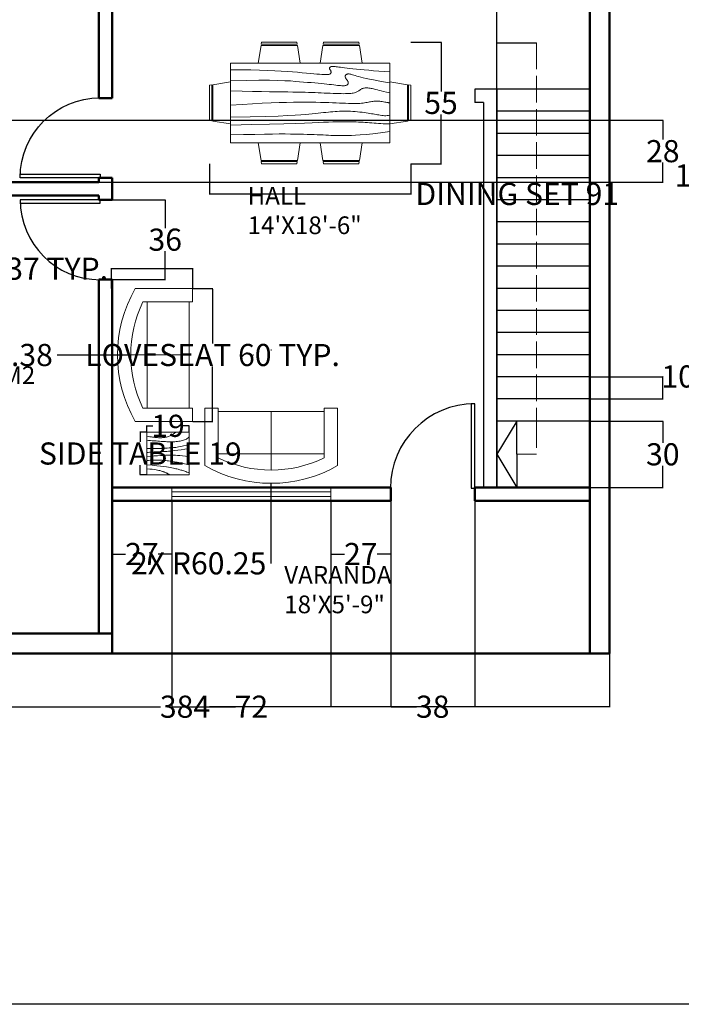
# Model space of a CAD drawing. Units: inches. Extents: x -16 to 1298, y 3 to 744.
# Tile 2 of 5: x 221 to 520, y 3 to 448. Entities that reach past the tile are written whole.
import ezdxf

# ---------------------------------------------------------------- set-up
doc = ezdxf.new("R2010")
doc.units = ezdxf.units.IN
doc.header["$MEASUREMENT"] = 0
doc.linetypes.add('ACAD_ISO02W100', pattern=[15, 12, -3])
for name, color, linetype, lineweight in [('A-ANNO-DIMS', 2, 'Continuous', 18), ('A-AREA-IDEN', 7, 'Continuous', 18), ('A-DOOR', 3, 'Continuous', 25), ('A-FLOR-STRS', 7, 'Continuous', 25), ('A-FLOR-STRS-PATH', 2, 'ACAD_ISO02W100', 13), ('A-FURN', 8, 'Continuous', 18), ('A-GLAZ', 4, 'Continuous', 18), ('A-WALL', 7, 'Continuous', 50)]:
    doc.layers.add(name, color=color, linetype=linetype, lineweight=lineweight)
doc.styles.get("Standard").update_dxf_attribs({"font": 'arial.ttf'})
doc.dimstyles.get("Standard").update_dxf_attribs({"dimtxt": 10, "dimasz": 0.18, "dimexe": 0.18, "dimexo": 0.0625, "dimgap": 0.09, "dimtad": 0, "dimtih": 1, "dimtoh": 1, "dimdec": 0, "dimzin": 0, "dimdsep": 46, "dimlunit": 3, "dimtxsty": 'Standard', "dimcen": 0.09, "dimadec": 0, "dimazin": 0, "dimtfac": 1, "dimtdec": 0, "dimtofl": 0, "dimtmove": 0, "dimatfit": 3, "dimfxl": 1, "dimtolj": 1, "dimtzin": 0, "dimarcsym": 0})

# ---------------------------------------------------------------- blocks, each defined once
blk = doc.blocks.new('Sofa - Roundback Loveseat 5 ft.')
for p, q in [((0, -32.44198), (0, -5.99998)), ((-24, -33.99998), (-24, -11.46958)), ((24.00004, -33.99998), (24.00004, -11.46958)), ((-23.9998, -13.38178), (23.99986, -13.38178)), ((-24, -32.44198), (24.00004, -32.44198))]:
    blk.add_line(p, q)
for points in [[(-24, -33.99998), (-30, -33.99998), (-30, -7.99998)], [(30.00004, -7.99998), (30.00004, -33.99998), (24.00004, -33.99998)]]:
    blk.add_lwpolyline(points)
for centre, radius, start, end in [((0, -60.24998), 60.24998, 60.13715, 119.8628), ((0, -61.38438), 55.38444, 64.32083, 115.6792)]:
    blk.add_arc(centre, radius, start, end)
blk = doc.blocks.new('Dining Set - 36 x 72 in.')
for p, q in [((-22, 27.5), (-22.1562, 26.50042)), ((-22, 27.5), (-6, 27.5)), ((-5.8437, 26.49966), (-6, 27.5)), ((6, 27.5), (5.8438, 26.50042)), ((6, 27.5), (22, 27.5)), ((22.1563, 26.49966), (22, 27.5)), ((-22.2343, 26.00059), (-23.4847, 17.99762)), ((-22.2304, 26), (-5.7608, 26)), ((-5.8416, 26.5), (-22.1534, 26.5)), ((-4.5152, 17.99762), (-5.7655, 25.99926)), ((5.7657, 26.00059), (4.5153, 17.99762)), ((5.7696, 26), (22.2392, 26)), ((22.1584, 26.5), (5.8466, 26.5)), ((23.4848, 17.99762), (22.2345, 25.99926)), ((36, 18), (-36, 18)), ((-36, 18), (-36, -18)), ((36, -18), (36, 18)), ((-44.0006, 8.23428), (-35.9976, 9.48474)), ((44.0006, 8.23428), (35.9976, 9.48474)), ((-45.5, 8), (-44.5004, 8.15617)), ((-45.5, 8), (-45.5, -8)), ((-44.5, -8.15843), (-44.5, 8.15338)), ((-44, 8.23041), (-44, -8.23915)), ((44, 8.23041), (44, -8.23915)), ((44.5, -8.15843), (44.5, 8.15338)), ((45.5, 8), (44.5005, 8.15617)), ((45.5, 8), (45.5, -8)), ((-44.4997, -8.15631), (-45.5, -8)), ((-35.9976, -9.48476), (-43.9993, -8.2345)), ((35.9976, -9.48476), (43.9993, -8.2345)), ((44.4997, -8.15631), (45.5, -8)), ((-36, -18), (36, -18)), ((-22.2343, -26.0006), (-23.4847, -17.99762)), ((-4.5152, -17.99762), (-5.7655, -25.99928)), ((5.7657, -26.0006), (4.5153, -17.99762)), ((23.4848, -17.99762), (22.2345, -25.99928)), ((-22.2304, -26), (-5.7608, -26)), ((-22, -27.5), (-22.1562, -26.50044)), ((-5.8416, -26.5), (-22.1534, -26.5)), ((-5.8437, -26.49967), (-6, -27.5)), ((5.7696, -26), (22.2392, -26)), ((6, -27.5), (5.8438, -26.50044)), ((22.1584, -26.5), (5.8466, -26.5)), ((22.1563, -26.49967), (22, -27.5)), ((-22, -27.5), (-6, -27.5)), ((6, -27.5), (22, -27.5))]:
    blk.add_line(p, q)
for points in [[(-36, 15), (-31.1772, 14.97754), (-26.8079, 14.91406), (-22.8538, 14.81543), (-19.276, 14.6875), (-16.0362, 14.53613), (-13.0957, 14.36718), (-10.4159, 14.18652), (-7.9583, 14), (-5.6904, 13.81315), (-3.6035, 13.63021), (-1.6954, 13.45508), (0.0365, 13.29166), (1.5945, 13.14388), (2.9811, 13.01562), (4.1988, 12.9108), (5.25, 12.83333), (6.1393, 12.78613), (6.8802, 12.76823), (7.4883, 12.77767), (7.9792, 12.8125), (8.3685, 12.87077), (8.6719, 12.95052), (8.9049, 13.0498), (9.0833, 13.16666), (9.2205, 13.29899), (9.3216, 13.44401), (9.3895, 13.59879), (9.4271, 13.76041), (9.4373, 13.92594), (9.4232, 14.09245), (9.3875, 14.257), (9.3333, 14.41666), (9.2638, 14.56917), (9.1836, 14.71484), (9.0975, 14.85465), (9.0104, 14.98958), (8.9272, 15.1206), (8.8529, 15.2487), (8.7922, 15.37483), (8.75, 15.5), (8.7305, 15.62467), (8.7344, 15.74739), (8.7617, 15.86621), (8.8125, 15.97916), (8.8867, 16.08431), (8.9844, 16.17968), (9.1055, 16.26334), (9.25, 16.33333), (9.4189, 16.38802), (9.6172, 16.42708), (9.8506, 16.45052), (10.125, 16.45833), (10.4463, 16.45052), (10.8203, 16.42708), (11.2529, 16.38802), (11.75, 16.33333), (12.3184, 16.26318), (12.9694, 16.17838), (13.7151, 16.07991), (14.5677, 15.96875), (15.5395, 15.84586), (16.6426, 15.71224), (17.8893, 15.56884), (19.2917, 15.41666), (20.859, 15.25667), (22.5879, 15.08984), (24.4721, 14.91715), (26.5052, 14.73958), (28.6809, 14.5581), (30.9929, 14.3737), (33.4347, 14.18733), (36, 14)], [(-36, 10), (-28.9766, 10.14274), (-23.1725, 10.20442), (-18.4241, 10.19775), (-14.5677, 10.13541), (-11.4399, 10.03011), (-8.877, 9.89453), (-6.7154, 9.74137), (-4.7917, 9.58333), (-2.9698, 9.43082), (-1.2246, 9.28515), (0.4415, 9.14534), (2.026, 9.01041), (3.5266, 8.87939), (4.9408, 8.7513), (6.266, 8.62516), (7.5, 8.5), (8.6411, 8.37549), (9.6914, 8.2539), (10.6538, 8.13818), (11.5312, 8.03125), (12.3267, 7.93603), (13.043, 7.85547), (13.6831, 7.79248), (14.25, 7.75), (14.7471, 7.7303), (15.1797, 7.73307), (15.5537, 7.75732), (15.875, 7.80208), (16.1494, 7.86637), (16.3828, 7.94922), (16.5811, 8.04964), (16.75, 8.16666), (16.8944, 8.29915), (17.0143, 8.44531), (17.1089, 8.60319), (17.1771, 8.77083), (17.218, 8.94629), (17.2305, 9.1276), (17.2137, 9.31282), (17.1667, 9.5), (17.0895, 9.6875), (16.987, 9.875), (16.8649, 10.0625), (16.7292, 10.25), (16.5856, 10.4375), (16.4401, 10.625), (16.2985, 10.8125), (16.1667, 11), (16.05, 11.18733), (15.9518, 11.3737), (15.8752, 11.5581), (15.8229, 11.73958), (15.798, 11.91715), (15.8034, 12.08984), (15.842, 12.25667), (15.9167, 12.41666), (16.0295, 12.56836), (16.1784, 12.70833), (16.3605, 12.83268), (16.5729, 12.9375), (16.8127, 13.01888), (17.0768, 13.07291), (17.3625, 13.0957), (17.6667, 13.08333), (17.9894, 13.03312), (18.3418, 12.94726), (18.7382, 12.82918), (19.1927, 12.68229), (19.7195, 12.51001), (20.3327, 12.31575), (21.0465, 12.10294), (21.875, 11.875), (22.8357, 11.63354), (23.959, 11.37304), (25.2786, 11.08618), (26.8282, 10.76562), (28.6414, 10.40405), (30.752, 9.99414), (33.1936, 9.52856), (36, 9)], [(-36, 5.5), (-30.7157, 5.3348), (-26.069, 5.20963), (-21.9946, 5.11767), (-18.4271, 5.05208), (-15.3009, 5.00602), (-12.5508, 4.97265), (-10.1112, 4.94515), (-7.9167, 4.91666), (-5.909, 4.88167), (-4.0586, 4.83984), (-2.3429, 4.79215), (-0.7396, 4.73958), (0.7739, 4.6831), (2.22, 4.6237), (3.6213, 4.56233), (5, 4.5), (6.373, 4.43782), (7.7344, 4.3776), (9.0723, 4.32129), (10.375, 4.27083), (11.6309, 4.22819), (12.8281, 4.19531), (13.9551, 4.17415), (15, 4.16666), (15.954, 4.17448), (16.819, 4.19791), (17.6001, 4.23698), (18.3021, 4.29166), (18.9299, 4.36198), (19.4883, 4.44791), (19.9823, 4.54948), (20.4167, 4.66666), (20.7969, 4.79899), (21.1302, 4.94401), (21.4245, 5.09879), (21.6875, 5.26041), (21.9271, 5.42594), (22.1511, 5.59245), (22.3672, 5.757), (22.5834, 5.91666), (22.8065, 6.06868), (23.0404, 6.21093), (23.2879, 6.34147), (23.5521, 6.45833), (23.8358, 6.55957), (24.142, 6.64323), (24.4735, 6.70735), (24.8334, 6.75), (25.2235, 6.76969), (25.642, 6.76692), (26.0858, 6.74267), (26.5521, 6.69791), (27.0379, 6.63362), (27.5404, 6.55078), (28.0565, 6.45036), (28.5834, 6.33333), (29.1242, 6.19987), (29.7071, 6.04687), (30.3661, 5.87044), (31.1354, 5.66666), (32.0493, 5.43164), (33.142, 5.16146), (34.4475, 4.85221), (36, 4.5)], [(-36, -1), (-30.7915, -0.6591), (-26.0195, -0.38216), (-21.6519, -0.16284), (-17.6563, 0.00521), (-14.0005, 0.12833), (-10.6523, 0.21289), (-7.5796, 0.26522), (-4.75, 0.29166), (-2.134, 0.29793), (0.2878, 0.28711), (2.5317, 0.26163), (4.6146, 0.22396), (6.5529, 0.17651), (8.3633, 0.12174), (10.0623, 0.06209), (11.6667, 0), (13.1899, -0.06201), (14.6341, -0.1211), (15.9982, -0.17432), (17.2813, -0.21875), (18.4823, -0.25147), (19.6003, -0.26953), (20.6343, -0.27002), (21.5834, -0.25), (22.4481, -0.20768), (23.2357, -0.14584), (23.9549, -0.06836), (24.6146, 0.02083), (25.2235, 0.11784), (25.7904, 0.21875), (26.3241, 0.31966), (26.8334, 0.41666), (27.3265, 0.50618), (27.8099, 0.58593), (28.2894, 0.65397), (28.7709, 0.70833), (29.2601, 0.74707), (29.763, 0.76823), (30.2855, 0.76985), (30.8334, 0.75), (31.4088, 0.70784), (31.9994, 0.64713), (32.589, 0.57275), (33.1615, 0.48958), (33.7008, 0.4025), (34.1908, 0.3164), (34.6153, 0.23616), (34.9584, 0.16666), (35.2099, 0.11165), (35.3848, 0.07031), (35.504, 0.04069), (35.5886, 0.02083), (35.6594, 0.00879), (35.7377, 0.0026), (35.8442, 0.00032), (36, 0)], [(-36, -6.5), (-27.1843, -6.31267), (-20.084, -6.1263), (-14.469, -5.9419), (-10.1094, -5.76042), (-6.7752, -5.58285), (-4.2363, -5.41016), (-2.2629, -5.24333), (-0.625, -5.08334), (0.8708, -4.93099), (2.2715, -4.78646), (3.5872, -4.64974), (4.8281, -4.52084), (6.0046, -4.39974), (7.127, -4.28646), (8.2053, -4.18099), (9.25, -4.08334), (10.2705, -3.99382), (11.2734, -3.91407), (12.2647, -3.84603), (13.25, -3.79167), (14.2354, -3.75293), (15.2266, -3.73177), (16.2295, -3.73015), (17.25, -3.75), (18.2912, -3.79248), (19.3451, -3.85547), (20.4009, -3.93604), (21.4479, -4.03125), (22.4754, -4.13819), (23.4727, -4.25391), (24.4289, -4.37549), (25.3334, -4.5), (26.1785, -4.62492), (26.9694, -4.74935), (27.7145, -4.87281), (28.4219, -4.99479), (29.1, -5.11483), (29.7572, -5.23242), (30.4016, -5.34709), (31.0417, -5.45834), (31.6837, -5.56437), (32.3262, -5.65821), (32.9658, -5.73153), (33.599, -5.77604), (34.2224, -5.78345), (34.8327, -5.74545), (35.4264, -5.65373), (36, -5.5)], [(-36, -10), (-26.4022, -9.81299), (-18.4675, -9.62891), (-11.9839, -9.45069), (-6.7396, -9.28125), (-2.5226, -9.12354), (0.8789, -8.98047), (3.6769, -8.85498), (6.0833, -8.75), (8.2767, -8.66765), (10.3021, -8.60677), (12.1712, -8.56543), (13.8958, -8.54167), (15.4876, -8.53353), (16.9583, -8.53907), (18.3197, -8.55632), (19.5834, -8.58334), (20.7616, -8.61841), (21.8685, -8.66081), (22.9188, -8.71004), (23.9271, -8.76563), (24.9081, -8.82707), (25.8763, -8.89388), (26.8465, -8.96558), (27.8334, -9.04167), (28.8474, -9.12118), (29.8828, -9.20117), (30.93, -9.27824), (31.9792, -9.34896), (33.0205, -9.40991), (34.0443, -9.45768), (35.0407, -9.48885), (36, -9.5)], [(-36, -14.5), (-30.0881, -14.33513), (-25.0332, -14.21224), (-20.7312, -14.12647), (-17.0781, -14.07292), (-13.97, -14.04671), (-11.3027, -14.04297), (-8.9724, -14.05681), (-6.875, -14.08334), (-4.9224, -14.11833), (-3.0905, -14.16016), (-1.3709, -14.20785), (0.2448, -14.26042), (1.7647, -14.3169), (3.1973, -14.3763), (4.5507, -14.43767), (5.8333, -14.5), (7.0554, -14.5621), (8.235, -14.62175), (9.3922, -14.67652), (10.5469, -14.72396), (11.7192, -14.76164), (12.929, -14.78711), (14.1965, -14.79794), (15.5417, -14.79167), (16.9933, -14.76424), (18.6152, -14.70508), (20.4804, -14.60197), (22.6615, -14.44271), (25.2312, -14.21509), (28.2624, -13.9069), (31.8277, -13.50594), (36, -13)]]:
    blk.add_lwpolyline(points)
blk = doc.blocks.new('*U8')
for p, q in [((0, 0), (0, -6)), ((-40, 0), (-40, -6))]:
    blk.add_line(p, q)
blk.add_lwpolyline([(0, 0), (0, 40), (-1.75, 40), (-1.75, 0)], close=True)
blk.add_arc((0, 0), 40, 90, 180)
blk = doc.blocks.new('Table - Square Woodgrain 42 x 42 in.')
blk.add_line((0, -42), (42, -42))
for points in [[(0, -4), (1.704, -4.2172), (3.2358, -4.4188), (4.615, -4.604), (5.8615, -4.7721), (6.9951, -4.9224), (8.0357, -5.0541), (9.0031, -5.1667), (9.9171, -5.2594), (10.7951, -5.3316), (11.6445, -5.3836), (12.4702, -5.4157), (13.277, -5.4283), (14.0698, -5.4217), (14.8535, -5.3964), (15.6331, -5.3526), (16.4133, -5.2908), (17.1986, -5.2103), (17.9913, -5.1062), (18.793, -4.9727), (19.6056, -4.8038), (20.4307, -4.5937), (21.2701, -4.3365), (22.1256, -4.0262), (22.9989, -3.6571), (23.888, -3.2272), (24.7756, -2.7516), (25.6408, -2.2491), (26.4624, -1.7387), (27.2195, -1.2395), (27.891, -0.7703), (28.456, -0.3501), (28.8934, 0.002)], [(0, -42), (0, 0), (42, 0), (42, -42)], [(0, -8), (1.8203, -8.1001), (3.6741, -8.2149), (5.5411, -8.3408), (7.4011, -8.4741), (9.2339, -8.6112), (11.0193, -8.7484), (12.7371, -8.8821), (14.3671, -9.0086), (15.8954, -9.1246), (17.3337, -9.2278), (18.6997, -9.3159), (20.0116, -9.387), (21.2871, -9.4389), (22.5442, -9.4696), (23.8008, -9.477), (25.0749, -9.459), (26.3791, -9.4137), (27.7049, -9.3403), (29.0383, -9.2382), (30.3655, -9.1068), (31.6728, -8.9455), (32.9461, -8.7535), (34.1717, -8.5304), (35.3358, -8.2756), (36.4268, -7.9863), (37.443, -7.6521), (38.3849, -7.2603), (39.253, -6.7986), (40.048, -6.2542), (40.7705, -5.6147), (41.421, -4.8674), (42, -4)], [(42, -12), (39.1784, -12.8621), (36.4519, -13.5654), (33.8246, -14.1294), (31.3004, -14.5731), (28.8832, -14.9161), (26.577, -15.1775), (24.3858, -15.3768), (22.3136, -15.5332), (20.3622, -15.6632), (18.5254, -15.7718), (16.7947, -15.8612), (15.1618, -15.9338), (13.6183, -15.9916), (12.1558, -16.0369), (10.7659, -16.0718), (9.4403, -16.0987), (8.1703, -16.1191), (6.9461, -16.1325), (5.7577, -16.1377), (4.595, -16.1335), (3.4479, -16.1188), (2.3064, -16.0924), (1.1604, -16.0532), (0, -16)], [(42, -16), (37.6529, -16.7365), (33.8802, -17.329), (30.6179, -17.7961), (27.8015, -18.1561), (25.3668, -18.4275), (23.2497, -18.6288), (21.3859, -18.7785), (19.7111, -18.8949), (18.1693, -18.9939), (16.7375, -19.0795), (15.401, -19.1534), (14.1449, -19.217), (12.9544, -19.2717), (11.8148, -19.3191), (10.7113, -19.3606), (9.6291, -19.3976), (8.5534, -19.4323), (7.47, -19.4689), (6.3643, -19.5122), (5.222, -19.5672), (4.0288, -19.6386), (2.7703, -19.7313), (1.4321, -19.8501), (0, -20)], [(0, -24), (3.9243, -23.6805), (7.4766, -23.4138), (10.6891, -23.1954), (13.5943, -23.0205), (16.2247, -22.8847), (18.6125, -22.7832), (20.7903, -22.7116), (22.7903, -22.6651), (24.6563, -22.642), (26.4764, -22.6507), (28.35, -22.7024), (30.3766, -22.8084), (32.6555, -22.98), (35.2861, -23.2283), (38.3678, -23.5645), (42, -24)], [(42, -32), (37.392, -31.017), (33.4585, -30.2231), (30.1291, -29.5949), (27.3334, -29.109), (25.0009, -28.742), (23.0612, -28.4707), (21.4439, -28.2716), (20.0786, -28.1215), (18.8998, -28.0002), (17.8609, -27.9014), (16.9206, -27.8219), (16.0371, -27.7588), (15.1691, -27.709), (14.2748, -27.6693), (13.3128, -27.6368), (12.2415, -27.6083), (11.0295, -27.5824), (9.6867, -27.5643), (8.233, -27.5608), (6.6884, -27.5787), (5.0728, -27.6248), (3.4062, -27.7058), (1.7086, -27.8286), (0, -28)], [(0, -32), (5.4026, -32.5358), (9.9494, -33.019), (13.7424, -33.4553), (16.8834, -33.8505), (19.4743, -34.2106), (21.6171, -34.5413), (23.4136, -34.8486), (24.9657, -35.1382), (26.3614, -35.4156), (27.6332, -35.6841), (28.7995, -35.9467), (29.8788, -36.2064), (30.8897, -36.4661), (31.8507, -36.7288), (32.7802, -36.9973), (33.6968, -37.2747), (34.6175, -37.5635), (35.5531, -37.8651), (36.5128, -38.1805), (37.506, -38.5108), (38.5421, -38.8568), (39.6302, -39.2197), (40.7797, -39.6004), (42, -40)], [(0, -36), (3.0098, -36.2857), (5.5354, -36.5643), (7.6368, -36.8359), (9.374, -37.1009), (10.807, -37.3597), (11.9957, -37.6126), (13.0002, -37.8599), (13.8804, -38.102), (14.6874, -38.3393), (15.4365, -38.5729), (16.1338, -38.8041), (16.7858, -39.0341), (17.3987, -39.264), (17.9787, -39.4952), (18.5322, -39.7288), (19.0655, -39.9662), (19.5832, -40.2081), (20.0842, -40.4544), (20.5657, -40.7046), (21.0249, -40.9581), (21.459, -41.2144), (21.8653, -41.4731), (22.2409, -41.7335), (22.5831, -41.9951)]]:
    blk.add_lwpolyline(points)
blk = doc.blocks.new('*D32')
at = {"layer": 'A-ANNO-DIMS', "color": 0, "lineweight": -2, "transparency": 16777216}
for p, q in [((299.2, 326.87), (308.32, 326.87)), ((308.14, 326.69), (308.14, 302.13)), ((308.14, 267.05), (308.14, 291.61)), ((299.2, 266.87), (308.32, 266.87))]:
    blk.add_line(p, q, dxfattribs=at)
at = {"layer": 'A-ANNO-DIMS', "color": 0, "transparency": 16777216}
for points in [[(308.11, 326.69), (308.17, 326.69), (308.14, 326.87)], [(308.11, 267.05), (308.17, 267.05), (308.14, 266.87)]]:
    blk.add_solid(points, dxfattribs=at)
at = {"layer": 'Defpoints', "color": 0, "transparency": 16777216}
for p in [(299.14, 326.87), (308.14, 326.87), (299.14, 266.87)]:
    blk.add_point(p, dxfattribs=at)
at = {"layer": 'A-ANNO-DIMS', "color": 0, "transparency": 16777216, "insert": (308.14, 296.87), "char_height": 10, "attachment_point": 5}
blk.add_mtext('\\A1;LOVESEAT 60 TYP.', dxfattribs=at)
blk = doc.blocks.new('*D33')
at = {"layer": 'A-ANNO-DIMS', "color": 0, "lineweight": -2, "transparency": 16777216}
for p, q in [((262.47, 335.87), (262.29, 335.87)), ((262.47, 326.93), (262.47, 336.05)), ((298.96, 335.87), (262.65, 335.87)), ((299.14, 326.93), (299.14, 336.05))]:
    blk.add_line(p, q, dxfattribs=at)
at = {"layer": 'A-ANNO-DIMS', "color": 0, "transparency": 16777216}
for points in [[(262.65, 335.9), (262.65, 335.84), (262.47, 335.87)], [(298.96, 335.9), (298.96, 335.84), (299.14, 335.87)]]:
    blk.add_solid(points, dxfattribs=at)
at = {"layer": 'Defpoints', "color": 0, "transparency": 16777216}
for p in [(262.47, 335.87), (262.47, 326.87), (299.14, 326.87)]:
    blk.add_point(p, dxfattribs=at)
at = {"layer": 'A-ANNO-DIMS', "color": 0, "transparency": 16777216, "insert": (237.87, 335.87), "char_height": 10, "attachment_point": 5}
blk.add_mtext('\\A1;37 TYP.', dxfattribs=at)
blk = doc.blocks.new('*D34')
at = {"layer": 'A-ANNO-DIMS', "color": 0, "lineweight": -2, "transparency": 16777216}
for p, q in [((278.28, 261.98), (275.28, 261.98)), ((275.46, 261.8), (275.46, 257.61)), ((275.46, 242.9), (275.46, 247.09)), ((278.28, 242.72), (275.28, 242.72))]:
    blk.add_line(p, q, dxfattribs=at)
at = {"layer": 'A-ANNO-DIMS', "color": 0, "transparency": 16777216}
for points in [[(275.43, 261.8), (275.49, 261.8), (275.46, 261.98)], [(275.43, 242.9), (275.49, 242.9), (275.46, 242.72)]]:
    blk.add_solid(points, dxfattribs=at)
at = {"layer": 'Defpoints', "color": 0, "transparency": 16777216}
for p in [(275.46, 261.98), (278.35, 261.98), (278.35, 242.72)]:
    blk.add_point(p, dxfattribs=at)
at = {"layer": 'A-ANNO-DIMS', "color": 0, "transparency": 16777216, "insert": (275.46, 252.35), "char_height": 10, "attachment_point": 5}
blk.add_mtext('\\A1;SIDE TABLE 19', dxfattribs=at)
blk = doc.blocks.new('*D35')
at = {"layer": 'A-ANNO-DIMS', "color": 0, "lineweight": -2, "transparency": 16777216}
for p, q in [((278.35, 262.04), (278.35, 265.05)), ((278.53, 264.87), (281.18, 264.87)), ((297.42, 264.87), (294.77, 264.87)), ((297.6, 262.04), (297.6, 265.05))]:
    blk.add_line(p, q, dxfattribs=at)
at = {"layer": 'A-ANNO-DIMS', "color": 0, "transparency": 16777216}
for points in [[(278.53, 264.9), (278.53, 264.84), (278.35, 264.87)], [(297.42, 264.9), (297.42, 264.84), (297.6, 264.87)]]:
    blk.add_solid(points, dxfattribs=at)
at = {"layer": 'Defpoints', "color": 0, "transparency": 16777216}
for p in [(297.6, 264.87), (278.35, 261.98), (297.6, 261.98)]:
    blk.add_point(p, dxfattribs=at)
at = {"layer": 'A-ANNO-DIMS', "color": 0, "transparency": 16777216, "insert": (287.97, 264.87), "char_height": 10, "attachment_point": 5}
blk.add_mtext('\\A1;19', dxfattribs=at)
blk = doc.blocks.new('*D36')
at = {"layer": 'A-ANNO-DIMS', "color": 0, "lineweight": -2, "transparency": 16777216}
for p, q in [((306.79, 383.23), (306.79, 369.47)), ((397.79, 383.23), (397.79, 369.47)), ((306.97, 369.65), (397.61, 369.65)), ((397.79, 369.65), (397.97, 369.65))]:
    blk.add_line(p, q, dxfattribs=at)
at = {"layer": 'A-ANNO-DIMS', "color": 0, "transparency": 16777216}
for points in [[(306.97, 369.68), (306.97, 369.62), (306.79, 369.65)], [(397.61, 369.68), (397.61, 369.62), (397.79, 369.65)]]:
    blk.add_solid(points, dxfattribs=at)
at = {"layer": 'Defpoints', "color": 0, "transparency": 16777216}
for p in [(306.79, 383.3), (397.79, 383.3), (397.79, 369.65)]:
    blk.add_point(p, dxfattribs=at)
at = {"layer": 'A-ANNO-DIMS', "color": 0, "transparency": 16777216, "insert": (445.92, 369.65), "char_height": 10, "attachment_point": 5}
blk.add_mtext('\\A1;DINING SET 91', dxfattribs=at)
blk = doc.blocks.new('*D37')
at = {"layer": 'A-ANNO-DIMS', "color": 0, "lineweight": -2, "transparency": 16777216}
for p, q in [((397.85, 438.3), (411.62, 438.3)), ((411.44, 438.12), (411.44, 415.97)), ((411.44, 383.48), (411.44, 405.62)), ((397.85, 383.3), (411.62, 383.3))]:
    blk.add_line(p, q, dxfattribs=at)
at = {"layer": 'A-ANNO-DIMS', "color": 0, "transparency": 16777216}
for points in [[(411.41, 438.12), (411.47, 438.12), (411.44, 438.3)], [(411.41, 383.48), (411.47, 383.48), (411.44, 383.3)]]:
    blk.add_solid(points, dxfattribs=at)
at = {"layer": 'Defpoints', "color": 0, "transparency": 16777216}
for p in [(397.79, 438.3), (411.44, 438.3), (397.79, 383.3)]:
    blk.add_point(p, dxfattribs=at)
at = {"layer": 'A-ANNO-DIMS', "color": 0, "transparency": 16777216, "insert": (411.44, 410.8), "char_height": 10, "attachment_point": 5}
blk.add_mtext('\\A1;55', dxfattribs=at)
blk = doc.blocks.new('*D40')
at = {"layer": 'A-ANNO-DIMS', "color": 0, "lineweight": -2, "transparency": 16777216}
for p, q in [((103.68, 161.93), (103.68, 137.76)), ((487.68, 161.93), (487.68, 137.76)), ((103.86, 137.94), (284.56, 137.94)), ((487.5, 137.94), (306.79, 137.94))]:
    blk.add_line(p, q, dxfattribs=at)
at = {"layer": 'A-ANNO-DIMS', "color": 0, "transparency": 16777216}
for points in [[(103.86, 137.97), (103.86, 137.91), (103.68, 137.94)], [(487.5, 137.97), (487.5, 137.91), (487.68, 137.94)]]:
    blk.add_solid(points, dxfattribs=at)
at = {"layer": 'Defpoints', "color": 0, "transparency": 16777216}
for p in [(103.68, 161.99), (487.68, 161.99), (487.68, 137.94)]:
    blk.add_point(p, dxfattribs=at)
at = {"layer": 'A-ANNO-DIMS', "color": 0, "transparency": 16777216, "insert": (295.68, 137.94), "char_height": 10, "attachment_point": 5}
blk.add_mtext('\\A1;384', dxfattribs=at)
blk = doc.blocks.new('*D42')
at = {"layer": 'A-ANNO-DIMS', "color": 0, "lineweight": -2, "transparency": 16777216}
for p, q in [((436.68, 237.05), (436.68, 618.22)), ((436.86, 618.04), (450.27, 618.04)), ((478.5, 618.04), (465.08, 618.04)), ((478.68, 237.05), (478.68, 618.22))]:
    blk.add_line(p, q, dxfattribs=at)
at = {"layer": 'A-ANNO-DIMS', "color": 0, "transparency": 16777216}
for points in [[(436.86, 618.07), (436.86, 618.01), (436.68, 618.04)], [(478.5, 618.07), (478.5, 618.01), (478.68, 618.04)]]:
    blk.add_solid(points, dxfattribs=at)
at = {"layer": 'Defpoints', "color": 0, "transparency": 16777216}
for p in [(478.68, 618.04), (436.68, 236.99), (478.68, 236.99)]:
    blk.add_point(p, dxfattribs=at)
at = {"layer": 'A-ANNO-DIMS', "color": 0, "transparency": 16777216, "insert": (457.68, 618.04), "char_height": 10, "attachment_point": 5}
blk.add_mtext('\\A1;42', dxfattribs=at)
blk = doc.blocks.new('*D43')
at = {"layer": 'A-ANNO-DIMS', "color": 0, "lineweight": -2, "transparency": 16777216}
for p, q in [((478.74, 266.99), (511.91, 266.99)), ((511.73, 266.81), (511.73, 257.19)), ((511.73, 237.17), (511.73, 246.79)), ((478.74, 236.99), (511.91, 236.99))]:
    blk.add_line(p, q, dxfattribs=at)
at = {"layer": 'A-ANNO-DIMS', "color": 0, "transparency": 16777216}
for points in [[(511.7, 266.81), (511.76, 266.81), (511.73, 266.99)], [(511.7, 237.17), (511.76, 237.17), (511.73, 236.99)]]:
    blk.add_solid(points, dxfattribs=at)
at = {"layer": 'Defpoints', "color": 0, "transparency": 16777216}
for p in [(478.68, 266.99), (511.73, 266.99), (478.68, 236.99)]:
    blk.add_point(p, dxfattribs=at)
at = {"layer": 'A-ANNO-DIMS', "color": 0, "transparency": 16777216, "insert": (511.73, 251.99), "char_height": 10, "attachment_point": 5}
blk.add_mtext('\\A1;30', dxfattribs=at)
blk = doc.blocks.new('*D44')
at = {"layer": 'A-ANNO-DIMS', "color": 0, "lineweight": -2, "transparency": 16777216}
for p, q in [((478.74, 286.99), (511.91, 286.99)), ((511.73, 286.99), (511.73, 287.17)), ((511.73, 287.17), (511.91, 287.17)), ((511.73, 277.17), (511.73, 286.81)), ((478.74, 276.99), (511.91, 276.99))]:
    blk.add_line(p, q, dxfattribs=at)
at = {"layer": 'A-ANNO-DIMS', "color": 0, "transparency": 16777216}
for points in [[(511.7, 286.81), (511.76, 286.81), (511.73, 286.99)], [(511.7, 277.17), (511.76, 277.17), (511.73, 276.99)]]:
    blk.add_solid(points, dxfattribs=at)
at = {"layer": 'Defpoints', "color": 0, "transparency": 16777216}
for p in [(478.68, 286.99), (511.73, 286.99), (478.68, 276.99)]:
    blk.add_point(p, dxfattribs=at)
at = {"layer": 'A-ANNO-DIMS', "color": 0, "transparency": 16777216, "insert": (518.67, 287.17), "char_height": 10, "attachment_point": 5}
blk.add_mtext('\\A1;10', dxfattribs=at)
blk = doc.blocks.new('*D49')
at = {"layer": 'A-ANNO-DIMS', "color": 0, "lineweight": -2, "transparency": 16777216}
for p, q in [((262.68, 230.93), (262.68, 206.76)), ((289.68, 230.93), (289.68, 206.76)), ((262.86, 206.94), (268.84, 206.94)), ((289.5, 206.94), (283.51, 206.94))]:
    blk.add_line(p, q, dxfattribs=at)
at = {"layer": 'A-ANNO-DIMS', "color": 0, "transparency": 16777216}
for points in [[(262.86, 206.97), (262.86, 206.91), (262.68, 206.94)], [(289.5, 206.97), (289.5, 206.91), (289.68, 206.94)]]:
    blk.add_solid(points, dxfattribs=at)
at = {"layer": 'Defpoints', "color": 0, "transparency": 16777216}
for p in [(262.68, 230.99), (289.68, 230.99), (262.68, 206.94)]:
    blk.add_point(p, dxfattribs=at)
at = {"layer": 'A-ANNO-DIMS', "color": 0, "transparency": 16777216, "insert": (276.18, 206.94), "char_height": 10, "attachment_point": 5}
blk.add_mtext('\\A1;27', dxfattribs=at)
blk = doc.blocks.new('*D50')
at = {"layer": 'A-ANNO-DIMS', "color": 0, "lineweight": -2, "transparency": 16777216}
for p, q in [((289.68, 230.93), (289.68, 137.76)), ((361.68, 230.93), (361.68, 137.76)), ((289.86, 137.94), (318.52, 137.94)), ((361.5, 137.94), (332.84, 137.94))]:
    blk.add_line(p, q, dxfattribs=at)
at = {"layer": 'A-ANNO-DIMS', "color": 0, "transparency": 16777216}
for points in [[(289.86, 137.97), (289.86, 137.91), (289.68, 137.94)], [(361.5, 137.97), (361.5, 137.91), (361.68, 137.94)]]:
    blk.add_solid(points, dxfattribs=at)
at = {"layer": 'Defpoints', "color": 0, "transparency": 16777216}
for p in [(289.68, 230.99), (361.68, 230.99), (361.68, 137.94)]:
    blk.add_point(p, dxfattribs=at)
at = {"layer": 'A-ANNO-DIMS', "color": 0, "transparency": 16777216, "insert": (325.68, 137.94), "char_height": 10, "attachment_point": 5}
blk.add_mtext('\\A1;72', dxfattribs=at)
blk = doc.blocks.new('*D51')
at = {"layer": 'A-ANNO-DIMS', "color": 0, "lineweight": -2, "transparency": 16777216}
for p, q in [((361.68, 230.93), (361.68, 206.76)), ((388.68, 230.93), (388.68, 206.76)), ((361.86, 206.94), (367.84, 206.94)), ((388.5, 206.94), (382.51, 206.94))]:
    blk.add_line(p, q, dxfattribs=at)
at = {"layer": 'A-ANNO-DIMS', "color": 0, "transparency": 16777216}
for points in [[(361.86, 206.97), (361.86, 206.91), (361.68, 206.94)], [(388.5, 206.97), (388.5, 206.91), (388.68, 206.94)]]:
    blk.add_solid(points, dxfattribs=at)
at = {"layer": 'Defpoints', "color": 0, "transparency": 16777216}
for p in [(361.68, 230.99), (388.68, 230.99), (361.68, 206.94)]:
    blk.add_point(p, dxfattribs=at)
at = {"layer": 'A-ANNO-DIMS', "color": 0, "transparency": 16777216, "insert": (375.18, 206.94), "char_height": 10, "attachment_point": 5}
blk.add_mtext('\\A1;27', dxfattribs=at)
blk = doc.blocks.new('*D52')
at = {"layer": 'A-ANNO-DIMS', "color": 0, "lineweight": -2, "transparency": 16777216}
for p, q in [((388.68, 230.93), (388.68, 137.76)), ((426.68, 230.93), (426.68, 137.76)), ((388.86, 137.94), (400.42, 137.94)), ((426.5, 137.94), (414.94, 137.94))]:
    blk.add_line(p, q, dxfattribs=at)
at = {"layer": 'A-ANNO-DIMS', "color": 0, "transparency": 16777216}
for points in [[(388.86, 137.97), (388.86, 137.91), (388.68, 137.94)], [(426.5, 137.97), (426.5, 137.91), (426.68, 137.94)]]:
    blk.add_solid(points, dxfattribs=at)
at = {"layer": 'Defpoints', "color": 0, "transparency": 16777216}
for p in [(388.68, 230.99), (426.68, 230.99), (426.68, 137.94)]:
    blk.add_point(p, dxfattribs=at)
at = {"layer": 'A-ANNO-DIMS', "color": 0, "transparency": 16777216, "insert": (407.68, 137.94), "char_height": 10, "attachment_point": 5}
blk.add_mtext('\\A1;38', dxfattribs=at)
blk = doc.blocks.new('*D54')
at = {"layer": 'A-ANNO-DIMS', "color": 0, "lineweight": -2, "transparency": 16777216}
for p, q in [((262.74, 366.99), (286.91, 366.99)), ((286.73, 366.81), (286.73, 354.19)), ((286.73, 331.17), (286.73, 343.79)), ((262.74, 330.99), (286.91, 330.99))]:
    blk.add_line(p, q, dxfattribs=at)
at = {"layer": 'A-ANNO-DIMS', "color": 0, "transparency": 16777216}
for points in [[(286.7, 366.81), (286.76, 366.81), (286.73, 366.99)], [(286.7, 331.17), (286.76, 331.17), (286.73, 330.99)]]:
    blk.add_solid(points, dxfattribs=at)
at = {"layer": 'Defpoints', "color": 0, "transparency": 16777216}
for p in [(262.68, 366.99), (262.68, 330.99), (286.73, 330.99)]:
    blk.add_point(p, dxfattribs=at)
at = {"layer": 'A-ANNO-DIMS', "color": 0, "transparency": 16777216, "insert": (286.73, 348.99), "char_height": 10, "attachment_point": 5}
blk.add_mtext('\\A1;36', dxfattribs=at)
blk = doc.blocks.new('*D62')
at = {"layer": 'A-ANNO-DIMS', "color": 0, "lineweight": -2, "transparency": 16777216}
for p, q in [((159.46, 402.99), (511.91, 402.99)), ((511.73, 402.81), (511.73, 394.18)), ((511.73, 375.17), (511.73, 383.79)), ((169.96, 374.99), (511.91, 374.99))]:
    blk.add_line(p, q, dxfattribs=at)
at = {"layer": 'A-ANNO-DIMS', "color": 0, "transparency": 16777216}
for points in [[(511.7, 402.81), (511.76, 402.81), (511.73, 402.99)], [(511.7, 375.17), (511.76, 375.17), (511.73, 374.99)]]:
    blk.add_solid(points, dxfattribs=at)
at = {"layer": 'Defpoints', "color": 0, "transparency": 16777216}
for p in [(159.4, 402.99), (511.73, 402.99), (169.9, 374.99)]:
    blk.add_point(p, dxfattribs=at)
at = {"layer": 'A-ANNO-DIMS', "color": 0, "transparency": 16777216, "insert": (511.73, 388.99), "char_height": 10, "attachment_point": 5}
blk.add_mtext('\\A1;28', dxfattribs=at)
blk = doc.blocks.new('*D70')
at = {"layer": 'A-ANNO-DIMS', "color": 0, "lineweight": -2, "transparency": 16777216}
for p, q in [((669.47, 437.99), (528.28, 437.99)), ((528.46, 437.81), (528.46, 383.18)), ((528.46, 318.17), (528.46, 372.79)), ((720.47, 317.99), (528.28, 317.99))]:
    blk.add_line(p, q, dxfattribs=at)
at = {"layer": 'A-ANNO-DIMS', "color": 0, "transparency": 16777216}
for points in [[(528.43, 437.81), (528.49, 437.81), (528.46, 437.99)], [(528.43, 318.17), (528.49, 318.17), (528.46, 317.99)]]:
    blk.add_solid(points, dxfattribs=at)
at = {"layer": 'Defpoints', "color": 0, "transparency": 16777216}
for p in [(528.46, 437.99), (669.53, 437.99), (720.53, 317.99)]:
    blk.add_point(p, dxfattribs=at)
at = {"layer": 'A-ANNO-DIMS', "color": 0, "transparency": 16777216, "insert": (528.46, 377.99), "char_height": 10, "attachment_point": 5}
blk.add_mtext('\\A1;120', dxfattribs=at)
blk = doc.blocks.new('*D87')
at = {"layer": 'A-ANNO-DIMS', "color": 0, "lineweight": -2, "transparency": 16777216}
for p, q in [((334.57, 299.13), (334.75, 299.13)), ((334.66, 299.04), (334.66, 299.22)), ((334.66, 202.73), (334.66, 238.7)), ((334.48, 202.73), (334.66, 202.73))]:
    blk.add_line(p, q, dxfattribs=at)
at = {"layer": 'A-ANNO-DIMS', "color": 0, "transparency": 16777216}
blk.add_solid([(334.63, 238.7), (334.69, 238.7), (334.66, 238.88)], dxfattribs=at)
at = {"layer": 'Defpoints', "color": 0, "transparency": 16777216}
for p in [(334.66, 299.13), (334.66, 238.88)]:
    blk.add_point(p, dxfattribs=at)
at = {"layer": 'A-ANNO-DIMS', "color": 0, "transparency": 16777216, "insert": (301.86, 202.73), "char_height": 10, "attachment_point": 5}
blk.add_mtext('\\A1;2X R60.25', dxfattribs=at)
blk = doc.blocks.new('*D88')
at = {"layer": 'A-ANNO-DIMS', "color": 0, "lineweight": -2, "transparency": 16777216}
for p, q in [((237.91, 296.87), (270.96, 296.87)), ((326.43, 296.87), (326.61, 296.87)), ((326.52, 296.78), (326.52, 296.96))]:
    blk.add_line(p, q, dxfattribs=at)
at = {"layer": 'A-ANNO-DIMS', "color": 0, "transparency": 16777216}
blk.add_solid([(270.96, 296.9), (270.96, 296.84), (271.14, 296.87)], dxfattribs=at)
at = {"layer": 'Defpoints', "color": 0, "transparency": 16777216}
for p in [(271.14, 296.87), (326.52, 296.87)]:
    blk.add_point(p, dxfattribs=at)
at = {"layer": 'A-ANNO-DIMS', "color": 0, "transparency": 16777216, "insert": (205.32, 296.87), "char_height": 10, "attachment_point": 5}
blk.add_mtext('\\A1;2X R55.38', dxfattribs=at)

msp = doc.modelspace()

# ---------------------------------------------------------------- linework, layer by layer
at = {"layer": 'A-FLOR-STRS'}
for p, q in [((436.6768, 416.9884), (436.6768, 458.9884)), ((436.6768, 437.9884), (454.6768, 437.9884)), ((478.6768, 416.9884), (426.6768, 416.9884)), ((426.6768, 416.9884), (426.6768, 410.9884)), ((436.6768, 416.9884), (436.6768, 236.9884)), ((430.6768, 410.9884), (426.6768, 410.9884)), ((430.6768, 410.9884), (430.6768, 236.9884)), ((478.6768, 406.9884), (436.6768, 406.9884)), ((478.6768, 396.9884), (436.6768, 396.9884)), ((478.6768, 386.9884), (436.6768, 386.9884)), ((478.6768, 376.9884), (436.6768, 376.9884)), ((478.6768, 366.9884), (436.6768, 366.9884)), ((478.6768, 356.9884), (436.6768, 356.9884)), ((478.6768, 346.9884), (436.6768, 346.9884)), ((478.6768, 336.9884), (436.6768, 336.9884)), ((478.6768, 326.9884), (436.6768, 326.9884)), ((478.6768, 316.9884), (436.6768, 316.9884)), ((478.6768, 306.9884), (436.6768, 306.9884)), ((478.6768, 296.9884), (436.6768, 296.9884)), ((478.6768, 286.9884), (436.6768, 286.9884)), ((478.6768, 276.9884), (436.6768, 276.9884)), ((478.6768, 266.9884), (436.6768, 266.9884)), ((436.6768, 266.9884), (436.6768, 236.9884)), ((445.6768, 266.9884), (436.6768, 251.9884)), ((445.6768, 251.9884), (445.6768, 266.9884)), ((436.6768, 251.9884), (445.6768, 236.9884)), ((445.6768, 251.9884), (445.6768, 236.9884))]:
    msp.add_line(p, q, dxfattribs=at)
at = {"layer": 'A-FLOR-STRS-PATH'}
for p, q in [((454.6768, 437.9884), (454.6768, 266.9884)), ((454.6768, 266.9884), (454.6768, 251.9884)), ((454.6768, 251.9884), (445.6768, 251.9884))]:
    msp.add_line(p, q, dxfattribs=at)
at = {"layer": 'A-GLAZ'}
for p, q in [((289.6768, 236.9884), (289.6768, 230.9884)), ((361.6768, 236.9884), (361.6768, 230.9884)), ((289.6768, 234.9884), (361.6768, 234.9884)), ((289.6768, 232.9884), (361.6768, 232.9884))]:
    msp.add_line(p, q, dxfattribs=at)
at = {"layer": 'A-WALL'}
for p, q in [((487.6768, 161.9884), (487.6768, 593.9884)), ((256.6768, 584.9884), (256.6768, 412.9884)), ((262.6768, 584.9884), (262.6768, 412.9884)), ((478.6768, 161.9884), (478.6768, 584.9884)), ((262.6768, 412.9884), (256.6768, 412.9884)), ((256.6768, 374.9884), (202.6768, 374.9884)), ((262.6768, 376.9884), (256.6768, 376.9884)), ((256.6768, 376.9884), (256.6768, 374.9884)), ((262.6768, 374.9884), (262.6768, 376.9884)), ((262.6768, 374.9884), (262.6768, 368.9884)), ((256.6768, 368.9884), (202.6768, 368.9884)), ((256.6768, 368.9884), (256.6768, 366.9884)), ((256.6768, 366.9884), (262.6768, 366.9884)), ((262.6768, 366.9884), (262.6768, 368.9884)), ((256.6768, 330.9884), (256.6768, 170.9884)), ((262.6768, 330.9884), (256.6768, 330.9884)), ((262.6768, 330.9884), (262.6768, 161.9884)), ((262.6768, 236.9884), (388.6768, 236.9884)), ((262.6768, 236.9884), (388.6768, 236.9884)), ((388.6768, 236.9884), (388.6768, 230.9884)), ((426.6768, 236.9884), (478.6768, 236.9884)), ((426.6768, 230.9884), (426.6768, 236.9884)), ((262.6768, 230.9884), (388.6768, 230.9884)), ((426.6768, 230.9884), (478.6768, 230.9884)), ((112.6768, 170.9884), (262.6768, 170.9884)), ((112.6768, 170.9884), (256.6768, 170.9884)), ((103.6768, 161.9884), (487.6768, 161.9884))]:
    msp.add_line(p, q, dxfattribs=at)
at = {"layer": 'Defpoints'}
msp.add_lwpolyline([(8.9336, 744.17), (1298.346, 744.17), (1298.346, 3.4476), (8.9336, 3.4476)], close=True, dxfattribs=at)

# ---------------------------------------------------------------- block references
at = {"layer": 'A-DOOR', "yscale": 0.9025287557699527, "zscale": 0.9025287557699527, "rotation": 90}
for p, xscale in [((257.2616, 376.9884), -0.9025287557699527), ((257.2616, 366.9884), 0.9025287557699527)]:
    msp.add_blockref('*U8', p, dxfattribs=dict(at, xscale=xscale))
at = {"layer": 'A-DOOR', "xscale": 0.9527312126739662, "yscale": 0.9527312126739662, "zscale": 0.9527312126739662}
msp.add_blockref('*U8', (426.6768, 236.7048), dxfattribs=at)
at = {"layer": 'A-FURN'}
msp.add_blockref('Dining Set - 36 x 72 in.', (352.286, 410.7963), dxfattribs=at)
for p, rotation in [((265.1378, 296.8707), 89.99999999999999), ((334.6572, 238.8789), 180)]:
    msp.add_blockref('Sofa - Roundback Loveseat 5 ft.', p, dxfattribs=dict(at, rotation=rotation))
at = {"layer": 'A-FURN', "xscale": 0.4584519016074886, "yscale": 0.4584519016074886, "zscale": 0.4584519016074886}
msp.add_blockref('Table - Square Woodgrain 42 x 42 in.', (278.3458, 261.9775), dxfattribs=at)

# ---------------------------------------------------------------- texts
at = {"layer": 'A-AREA-IDEN', "char_height": 8, "attachment_point": 1}
for s, insert in [('HALL\\P14\'X18\'-6"', (324.0015, 372.8361)), ("BEDROOM2\\P12'X11'", (168.8016, 291.7695)), ('VARANDA\\P18\'X5\'-9"', (340.5445, 201.5078))]:
    msp.add_mtext_dynamic_manual_height_columns(s, width=63.245227, gutter_width=1, heights=[0], dxfattribs=dict(at, insert=insert))

# ---------------------------------------------------------------- dimensions: what is measured, and where the dimension line sits
at = {"layer": 'A-ANNO-DIMS'}
for base, p1, p2, picture, middle in [((478.6768, 618.0384), (436.6768, 236.9884), (478.6768, 236.9884), '*D42', (457.6768, 618.0384)), ((297.6007, 264.8668), (278.3458, 261.9785), (297.6007, 261.9785), '*D35', (287.9732, 264.8668)), ((361.6768, 137.9384), (289.6768, 230.9884), (361.6768, 230.9884), '*D50', (325.6768, 137.9384)), ((426.6768, 137.9384), (388.6768, 230.9884), (426.6768, 230.9884), '*D52', (407.6768, 137.9384)), ((487.6768, 137.9384), (103.6768, 161.9884), (487.6768, 161.9884), '*D40', (295.6768, 137.9384))]:
    dim = msp.add_linear_dim(base=base, p1=p1, p2=p2, dimstyle='Standard', override={"dimdec": 0, "dimlfac": 1, "dimrnd": 0, "dimzin": 0, "dimdsep": 46, "dimlunit": 2}, dxfattribs=at)
    dim.commit()
    dim.dimension.update_dxf_attribs({"geometry": picture, "text_midpoint": middle})
for base, p1, p2, angle, picture, middle in [((411.436, 438.2963), (397.786, 383.2963), (397.786, 438.2963), 90, '*D37', (411.436, 410.7963)), ((528.4611, 437.9884), (720.5287, 317.9884), (669.5287, 437.9884), 90, '*D70', (528.4611, 377.9884)), ((511.7268, 402.9883), (169.8975, 374.9884), (159.3976, 402.9883), 90, '*D62', (511.7268, 388.9884)), ((286.7268, 330.9884), (262.6768, 366.9884), (262.6768, 330.9884), 270, '*D54', (286.7268, 348.9884)), ((511.7268, 286.9884), (478.6768, 276.9884), (478.6768, 286.9884), 90, '*D44', (518.6714, 287.1684)), ((511.7268, 266.9884), (478.6768, 236.9884), (478.6768, 266.9884), 90, '*D43', (511.7268, 251.9884)), ((262.6768, 206.9384), (289.6768, 230.9884), (262.6768, 230.9884), 180, '*D49', (276.1768, 206.9384)), ((361.6768, 206.9384), (388.6768, 230.9884), (361.6768, 230.9884), 180, '*D51', (375.1768, 206.9384))]:
    dim = msp.add_linear_dim(base=base, p1=p1, p2=p2, angle=angle, dimstyle='Standard', override={"dimdec": 0, "dimlfac": 1, "dimrnd": 0, "dimzin": 0, "dimdsep": 46, "dimlunit": 2}, dxfattribs=at)
    dim.commit()
    dim.dimension.update_dxf_attribs({"geometry": picture, "text_midpoint": middle})
dim = msp.add_linear_dim(base=(397.786, 369.6463), p1=(306.786, 383.2963), p2=(397.786, 383.2963), text='DINING SET <>', dimstyle='Standard', override={"dimdec": 0, "dimlfac": 1, "dimrnd": 0, "dimzin": 0, "dimdsep": 46, "dimlunit": 2}, dxfattribs=at)
dim.commit()
dim.dimension.update_dxf_attribs({"geometry": '*D36', "text_midpoint": (445.9175, 369.6463)})
for base, p1, p2, angle, text, picture, middle in [((262.4712, 335.8707), (299.1378, 326.8707), (262.4712, 326.8707), 180, '<> TYP.', '*D33', (237.8662, 335.8707)), ((308.1378, 326.8707), (299.1378, 266.8707), (299.1378, 326.8707), 90, 'LOVESEAT <> TYP.', '*D32', (308.1378, 296.8707)), ((275.4574, 261.9785), (278.3458, 242.7226), (278.3458, 261.9785), 90, 'SIDE TABLE <>', '*D34', (275.4574, 252.3505))]:
    dim = msp.add_linear_dim(base=base, p1=p1, p2=p2, angle=angle, text=text, dimstyle='Standard', override={"dimdec": 0, "dimlfac": 1, "dimrnd": 0, "dimzin": 0, "dimdsep": 46, "dimlunit": 2}, dxfattribs=at)
    dim.commit()
    dim.dimension.update_dxf_attribs({"geometry": picture, "text_midpoint": middle})
for center, mpoint, picture, middle in [((326.5222, 296.8707), (271.1378, 296.871), '*D88', (237.9071, 296.8712)), ((334.6572, 299.1288), (334.657, 238.8789), '*D87', (301.863, 202.7289))]:
    dim = msp.add_radius_dim(center=center, mpoint=mpoint, text='2X <>', dimstyle='Standard', override={"dimdec": 2, "dimlfac": 1, "dimrnd": 0, "dimzin": 0, "dimdsep": 46, "dimlunit": 2}, dxfattribs=at)
    dim.commit()
    dim.dimension.update_dxf_attribs({"geometry": picture, "text_midpoint": middle, "dimtype": 164})

doc.saveas('drawing.dxf')
